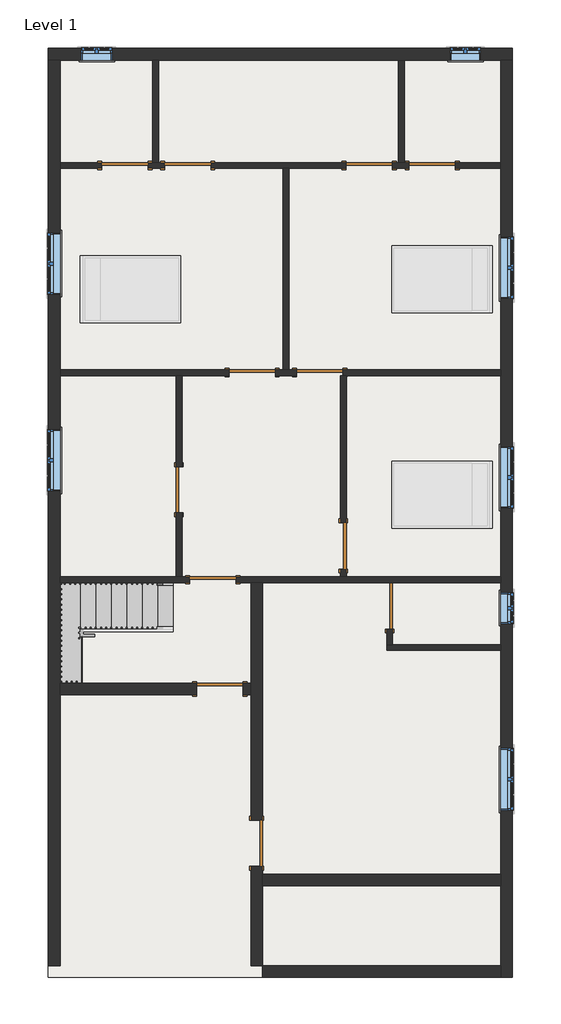
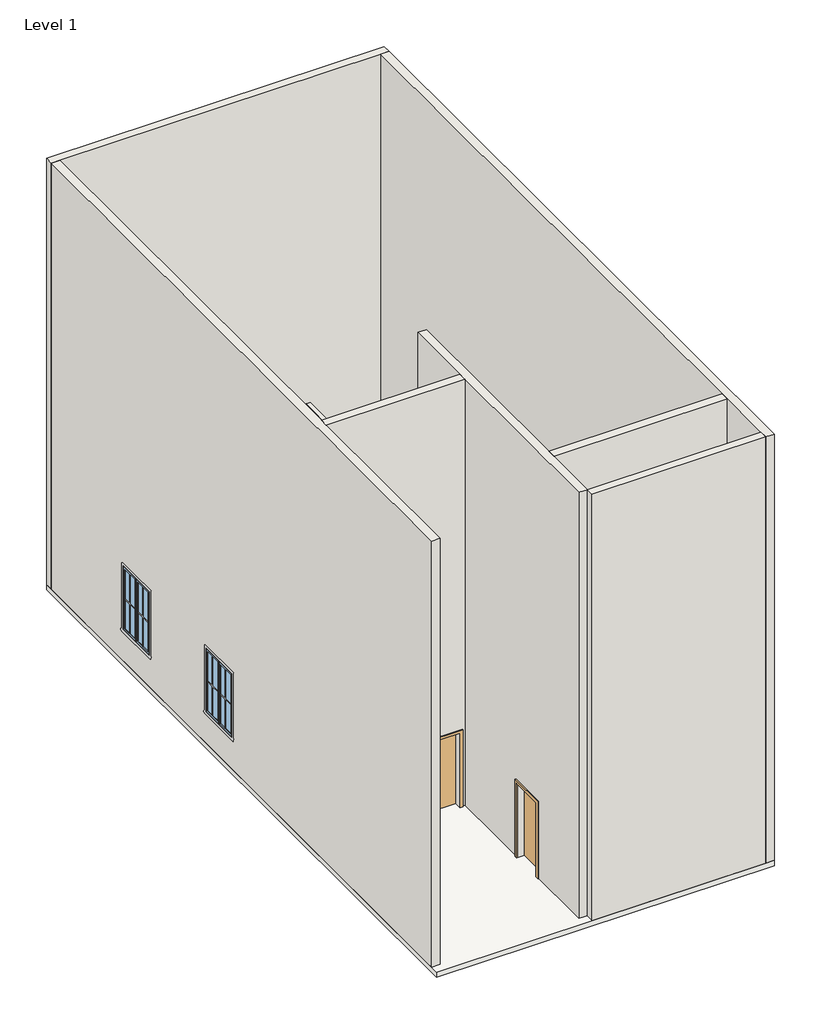
# One storey, part 1 of 2: 17 walls, 12 doors, 8 windows, 1 railing, 1 slab, 1 stair flight.
"""IFC4 building model written with IfcOpenShell, lengths in millimetres."""

from ifc_helpers import new_model, si_unit, frame, origin, origin_with_axes, place, context, project, spatial, polyline, outline, extrude, faceted_brep, transform, mapped, element, save
from components import door_305aa2a5, door_e5f9f3c4, door_0ca8825f, stair_flight_3e22188b, window_c417fced, window_6ca1769e

model = new_model("IFC4")

# Units and contexts
model_context = context("Model", 3, world=origin())
ifc_project = project(units=[si_unit("LENGTHUNIT", "METRE", prefix="MILLI")], contexts=[model_context])

# Site, building, storey
site = spatial("IfcSite", under=ifc_project)
building = spatial("IfcBuilding", under=site)
storey = spatial("IfcBuildingStorey", under=building, Name="Level 1", Elevation=0.0)

# Doors
placement = place(None, origin())
door_shape = door_305aa2a5(model_context)
element("IfcDoor", 1, ObjectType="Single-Flush : 36\" x 84\"", at=placement, inside=storey, context=model_context, shape_type="MappedRepresentation", body=[
    mapped(door_shape, transform((4013.2, 11918.95, 0.0), x_axis=(-1.0, 0.0, 0.0), y_axis=(0.0, -1.0, 0.0), z_axis=(0.0, 0.0, 1.0))),
])
element("IfcDoor", 2, ObjectType="Single-Flush : 36\" x 84\"", at=placement, inside=storey, context=model_context, shape_type="MappedRepresentation", body=[
    mapped(door_shape, transform((8832.85, 11918.95, 0.0), x_axis=(-1.0, 0.0, 0.0), y_axis=(0.0, -1.0, 0.0), z_axis=(0.0, 0.0, 1.0))),
])
element("IfcDoor", 3, ObjectType="Single-Flush : 36\" x 84\"", at=placement, inside=storey, context=model_context, shape_type="MappedRepresentation", body=[
    mapped(door_shape, transform((6616.7, 7842.25, 0.0), x_axis=(-1.0, 0.0, 0.0), y_axis=(0.0, -1.0, 0.0), z_axis=(0.0, 0.0, 1.0))),
])
element("IfcDoor", 4, ObjectType="Single-Flush : 36\" x 84\"", at=placement, inside=storey, context=model_context, shape_type="MappedRepresentation", body=[
    mapped(door_shape, transform((3841.75, 5537.2, 0.0), x_axis=(0.0, -1.0, 0.0), y_axis=(1.0, 0.0, 0.0), z_axis=(0.0, 0.0, 1.0))),
])
door_2_shape = door_e5f9f3c4(model_context)
element("IfcDoor", 5, ObjectType="Single-Flush : 36\" x 84\"", at=placement, inside=storey, context=model_context, shape_type="MappedRepresentation", body=[
    mapped(door_2_shape, transform((2774.95, 11918.95, 0.0), x_axis=(1.0, 0.0, 0.0), y_axis=(0.0, 1.0, 0.0), z_axis=(0.0, 0.0, 1.0))),
])
element("IfcDoor", 6, ObjectType="Single-Flush : 36\" x 84\"", at=placement, inside=storey, context=model_context, shape_type="MappedRepresentation", body=[
    mapped(door_2_shape, transform((7588.25, 11918.95, 0.0), x_axis=(1.0, 0.0, 0.0), y_axis=(0.0, 1.0, 0.0), z_axis=(0.0, 0.0, 1.0))),
])
element("IfcDoor", 7, ObjectType="Single-Flush : 36\" x 84\"", at=placement, inside=storey, context=model_context, shape_type="MappedRepresentation", body=[
    mapped(door_2_shape, transform((5283.2, 7842.25, 0.0), x_axis=(1.0, 0.0, 0.0), y_axis=(0.0, 1.0, 0.0), z_axis=(0.0, 0.0, 1.0))),
])
element("IfcDoor", 8, ObjectType="Single-Flush : 36\" x 84\"", at=placement, inside=storey, context=model_context, shape_type="MappedRepresentation", body=[
    mapped(door_2_shape, transform((4508.5, 3765.55, 0.0), x_axis=(1.0, 0.0, 0.0), y_axis=(0.0, 1.0, 0.0), z_axis=(0.0, 0.0, 1.0))),
])
element("IfcDoor", 9, ObjectType="Single-Flush : 36\" x 84\"", at=placement, inside=storey, context=model_context, shape_type="MappedRepresentation", body=[
    mapped(door_2_shape, transform((7080.25, 4432.3, 0.0), x_axis=(0.0, -1.0, 0.0), y_axis=(1.0, 0.0, 0.0), z_axis=(0.0, 0.0, 1.0))),
])
element("IfcDoor", 10, ObjectType="Single-Flush : 36\" x 84\"", at=placement, inside=storey, context=model_context, shape_type="MappedRepresentation", body=[
    mapped(door_2_shape, transform((7994.65, 3251.2, 0.0), x_axis=(0.0, -1.0, 0.0), y_axis=(1.0, 0.0, 0.0), z_axis=(0.0, 0.0, 1.0))),
])
door_3_shape = door_0ca8825f(model_context)
element("IfcDoor", 11, ObjectType="Single-Flush : 36\" x 84\"", at=placement, inside=storey, context=model_context, shape_type="MappedRepresentation", body=[
    mapped(door_3_shape, transform((4648.2, 1612.9, 0.0), x_axis=(1.0, 0.0, 0.0), y_axis=(0.0, 1.0, 0.0), z_axis=(0.0, 0.0, 1.0))),
])
element("IfcDoor", 12, ObjectType="Single-Flush : 36\" x 84\"", at=placement, inside=storey, context=model_context, shape_type="MappedRepresentation", body=[
    mapped(door_3_shape, transform((5372.1, -1422.4, 0.0), x_axis=(0.0, -1.0, 0.0), y_axis=(1.0, 0.0, 0.0), z_axis=(0.0, 0.0, 1.0))),
])

# Railing
element("IfcRailing", 13, ObjectType="Handrail - Rectangular", at=placement, inside=storey, context=model_context, shape_type="SolidModel", body=[
    faceted_brep([(3727.9146873, 3657.6, 1083.7333333), (3727.9146873, 3657.6, 1025.620221), (3727.9146873, 3708.4, 1025.620221), (3727.9146873, 3708.4, 1083.7333333), (1899.1146873, 3657.6, 2099.7333333), (1885.9510851, 3657.6, 2048.9333333), (1885.9510851, 3708.4, 2048.9333333), (1899.1146873, 3708.4, 2099.7333333), (1549.4, 3657.6, 2099.7333333), (1549.4, 3657.6, 2048.9333333), (1498.6, 3708.4, 2048.9333333), (1498.6, 3708.4, 2099.7333333), (1549.4, 1778.0, 2099.7333333), (1549.4, 1778.0, 2048.9333333), (1498.6, 1727.2, 2048.9333333), (1498.6, 1727.2, 2099.7333333), (1594.3146873, 1778.0, 2099.7333333), (1607.4782895, 1778.0, 2048.9333333), (1607.4782895, 1727.2, 2048.9333333), (1594.3146873, 1727.2, 2099.7333333), (3727.9146873, 1778.0, 3285.0666667), (3727.9146873, 1727.2, 3285.0666667), (3727.9146873, 1727.2, 3226.9535543), (3727.9146873, 1778.0, 3226.9535543)], [[[0, 1, 2, 3]], [[1, 0, 4, 5]], [[2, 1, 5, 6]], [[3, 2, 6, 7]], [[0, 3, 7, 4]], [[5, 4, 8, 9]], [[6, 5, 9, 10]], [[7, 6, 10, 11]], [[4, 7, 11, 8]], [[9, 8, 12, 13]], [[10, 9, 13, 14]], [[11, 10, 14, 15]], [[8, 11, 15, 12]], [[13, 12, 16, 17]], [[14, 13, 17, 18]], [[15, 14, 18, 19]], [[12, 15, 19, 16]], [[20, 21, 22, 23]], [[17, 16, 20, 23]], [[18, 17, 23, 22]], [[19, 18, 22, 21]], [[16, 19, 21, 20]]]),
    extrude(outline(polyline([(3193.1815058, 3667.125), (3182.5981725, 3648.075), (2201.3333333, 3648.075), (2201.3333333, 3667.125), (3193.1815058, 3667.125)])), frame((0.0, 1743.075, 0.0), z_axis=(0.0, 1.0, 0.0), x_axis=(0.0, 0.0, 1.0)), (0.0, 0.0, 1.0), 19.05),
    extrude(outline(polyline([(3136.7370614, 3565.525), (3126.153728, 3546.475), (2201.3333333, 3546.475), (2201.3333333, 3565.525), (3136.7370614, 3565.525)])), frame((0.0, 1743.075, 0.0), z_axis=(0.0, 1.0, 0.0), x_axis=(0.0, 0.0, 1.0)), (0.0, 0.0, 1.0), 19.05),
    extrude(outline(polyline([(3080.2926169, 3463.925), (3069.7092836, 3444.875), (2201.3333333, 3444.875), (2201.3333333, 3463.925), (3080.2926169, 3463.925)])), frame((0.0, 1743.075, 0.0), z_axis=(0.0, 1.0, 0.0), x_axis=(0.0, 0.0, 1.0)), (0.0, 0.0, 1.0), 19.05),
    extrude(outline(polyline([(3023.8481725, 3362.325), (3013.2648391, 3343.275), (2032.0, 3343.275), (2032.0, 3362.325), (3023.8481725, 3362.325)])), frame((0.0, 1743.075, 0.0), z_axis=(0.0, 1.0, 0.0), x_axis=(0.0, 0.0, 1.0)), (0.0, 0.0, 1.0), 19.05),
    extrude(outline(polyline([(2967.403728, 3260.725), (2956.8203947, 3241.675), (2032.0, 3241.675), (2032.0, 3260.725), (2967.403728, 3260.725)])), frame((0.0, 1743.075, 0.0), z_axis=(0.0, 1.0, 0.0), x_axis=(0.0, 0.0, 1.0)), (0.0, 0.0, 1.0), 19.05),
    extrude(outline(polyline([(2910.9592836, 3159.125), (2900.3759503, 3140.075), (2032.0, 3140.075), (2032.0, 3159.125), (2910.9592836, 3159.125)])), frame((0.0, 1743.075, 0.0), z_axis=(0.0, 1.0, 0.0), x_axis=(0.0, 0.0, 1.0)), (0.0, 0.0, 1.0), 19.05),
    extrude(outline(polyline([(2854.5148391, 3057.525), (2843.9315058, 3038.475), (1862.6666667, 3038.475), (1862.6666667, 3057.525), (2854.5148391, 3057.525)])), frame((0.0, 1743.075, 0.0), z_axis=(0.0, 1.0, 0.0), x_axis=(0.0, 0.0, 1.0)), (0.0, 0.0, 1.0), 19.05),
    extrude(outline(polyline([(2798.0703947, 2955.925), (2787.4870614, 2936.875), (1862.6666667, 2936.875), (1862.6666667, 2955.925), (2798.0703947, 2955.925)])), frame((0.0, 1743.075, 0.0), z_axis=(0.0, 1.0, 0.0), x_axis=(0.0, 0.0, 1.0)), (0.0, 0.0, 1.0), 19.05),
    extrude(outline(polyline([(2741.6259503, 2854.325), (2731.0426169, 2835.275), (1862.6666667, 2835.275), (1862.6666667, 2854.325), (2741.6259503, 2854.325)])), frame((0.0, 1743.075, 0.0), z_axis=(0.0, 1.0, 0.0), x_axis=(0.0, 0.0, 1.0)), (0.0, 0.0, 1.0), 19.05),
    extrude(outline(polyline([(2685.1815058, 2752.725), (2674.5981725, 2733.675), (1693.3333333, 2733.675), (1693.3333333, 2752.725), (2685.1815058, 2752.725)])), frame((0.0, 1743.075, 0.0), z_axis=(0.0, 1.0, 0.0), x_axis=(0.0, 0.0, 1.0)), (0.0, 0.0, 1.0), 19.05),
    extrude(outline(polyline([(2628.7370614, 2651.125), (2618.153728, 2632.075), (1693.3333333, 2632.075), (1693.3333333, 2651.125), (2628.7370614, 2651.125)])), frame((0.0, 1743.075, 0.0), z_axis=(0.0, 1.0, 0.0), x_axis=(0.0, 0.0, 1.0)), (0.0, 0.0, 1.0), 19.05),
    extrude(outline(polyline([(2572.2926169, 2549.525), (2561.7092836, 2530.475), (1693.3333333, 2530.475), (1693.3333333, 2549.525), (2572.2926169, 2549.525)])), frame((0.0, 1743.075, 0.0), z_axis=(0.0, 1.0, 0.0), x_axis=(0.0, 0.0, 1.0)), (0.0, 0.0, 1.0), 19.05),
    extrude(outline(polyline([(2515.8481725, 2447.925), (2505.2648391, 2428.875), (1524.0, 2428.875), (1524.0, 2447.925), (2515.8481725, 2447.925)])), frame((0.0, 1743.075, 0.0), z_axis=(0.0, 1.0, 0.0), x_axis=(0.0, 0.0, 1.0)), (0.0, 0.0, 1.0), 19.05),
    extrude(outline(polyline([(2459.403728, 2346.325), (2448.8203947, 2327.275), (1524.0, 2327.275), (1524.0, 2346.325), (2459.403728, 2346.325)])), frame((0.0, 1743.075, 0.0), z_axis=(0.0, 1.0, 0.0), x_axis=(0.0, 0.0, 1.0)), (0.0, 0.0, 1.0), 19.05),
    extrude(outline(polyline([(2402.9592836, 2244.725), (2392.3759503, 2225.675), (1524.0, 2225.675), (1524.0, 2244.725), (2402.9592836, 2244.725)])), frame((0.0, 1743.075, 0.0), z_axis=(0.0, 1.0, 0.0), x_axis=(0.0, 0.0, 1.0)), (0.0, 0.0, 1.0), 19.05),
    extrude(outline(polyline([(2346.5148391, 2143.125), (2335.9315058, 2124.075), (1354.6666667, 2124.075), (1354.6666667, 2143.125), (2346.5148391, 2143.125)])), frame((0.0, 1743.075, 0.0), z_axis=(0.0, 1.0, 0.0), x_axis=(0.0, 0.0, 1.0)), (0.0, 0.0, 1.0), 19.05),
    extrude(outline(polyline([(2290.0703947, 2041.525), (2279.4870614, 2022.475), (1354.6666667, 2022.475), (1354.6666667, 2041.525), (2290.0703947, 2041.525)])), frame((0.0, 1743.075, 0.0), z_axis=(0.0, 1.0, 0.0), x_axis=(0.0, 0.0, 1.0)), (0.0, 0.0, 1.0), 19.05),
    extrude(outline(polyline([(2233.6259503, 1939.925), (2223.0426169, 1920.875), (1354.6666667, 1920.875), (1354.6666667, 1939.925), (2233.6259503, 1939.925)])), frame((0.0, 1743.075, 0.0), z_axis=(0.0, 1.0, 0.0), x_axis=(0.0, 0.0, 1.0)), (0.0, 0.0, 1.0), 19.05),
    extrude(outline(polyline([(2177.1815058, 1838.325), (2166.5981725, 1819.275), (1185.3333333, 1819.275), (1185.3333333, 1838.325), (2177.1815058, 1838.325)])), frame((0.0, 1743.075, 0.0), z_axis=(0.0, 1.0, 0.0), x_axis=(0.0, 0.0, 1.0)), (0.0, 0.0, 1.0), 19.05),
    extrude(outline(polyline([(2120.7370614, 1736.725), (2110.153728, 1717.675), (1185.3333333, 1717.675), (1185.3333333, 1736.725), (2120.7370614, 1736.725)])), frame((0.0, 1743.075, 0.0), z_axis=(0.0, 1.0, 0.0), x_axis=(0.0, 0.0, 1.0)), (0.0, 0.0, 1.0), 19.05),
    extrude(outline(polyline([(2064.2926169, 1635.125), (2053.7092836, 1616.075), (1185.3333333, 1616.075), (1185.3333333, 1635.125), (2064.2926169, 1635.125)])), frame((0.0, 1743.075, 0.0), z_axis=(0.0, 1.0, 0.0), x_axis=(0.0, 0.0, 1.0)), (0.0, 0.0, 1.0), 19.05),
    extrude(outline(polyline([(1514.475, 1863.725), (1533.525, 1863.725), (1533.525, 1844.675), (1514.475, 1844.675), (1514.475, 1863.725)])), frame((0.0, 0.0, 1185.3333333), z_axis=(0.0, 0.0, 1.0), x_axis=(1.0, 0.0, 0.0)), (0.0, 0.0, 1.0), 863.6),
    extrude(outline(polyline([(1514.475, 1965.325), (1533.525, 1965.325), (1533.525, 1946.275), (1514.475, 1946.275), (1514.475, 1965.325)])), frame((0.0, 0.0, 1185.3333333), z_axis=(0.0, 0.0, 1.0), x_axis=(1.0, 0.0, 0.0)), (0.0, 0.0, 1.0), 863.6),
    extrude(outline(polyline([(1514.475, 2066.925), (1533.525, 2066.925), (1533.525, 2047.875), (1514.475, 2047.875), (1514.475, 2066.925)])), frame((0.0, 0.0, 1185.3333333), z_axis=(0.0, 0.0, 1.0), x_axis=(1.0, 0.0, 0.0)), (0.0, 0.0, 1.0), 863.6),
    extrude(outline(polyline([(1514.475, 2168.525), (1533.525, 2168.525), (1533.525, 2149.475), (1514.475, 2149.475), (1514.475, 2168.525)])), frame((0.0, 0.0, 1185.3333333), z_axis=(0.0, 0.0, 1.0), x_axis=(1.0, 0.0, 0.0)), (0.0, 0.0, 1.0), 863.6),
    extrude(outline(polyline([(1514.475, 2270.125), (1533.525, 2270.125), (1533.525, 2251.075), (1514.475, 2251.075), (1514.475, 2270.125)])), frame((0.0, 0.0, 1185.3333333), z_axis=(0.0, 0.0, 1.0), x_axis=(1.0, 0.0, 0.0)), (0.0, 0.0, 1.0), 863.6),
    extrude(outline(polyline([(1514.475, 2371.725), (1533.525, 2371.725), (1533.525, 2352.675), (1514.475, 2352.675), (1514.475, 2371.725)])), frame((0.0, 0.0, 1185.3333333), z_axis=(0.0, 0.0, 1.0), x_axis=(1.0, 0.0, 0.0)), (0.0, 0.0, 1.0), 863.6),
    extrude(outline(polyline([(1514.475, 2473.325), (1533.525, 2473.325), (1533.525, 2454.275), (1514.475, 2454.275), (1514.475, 2473.325)])), frame((0.0, 0.0, 1185.3333333), z_axis=(0.0, 0.0, 1.0), x_axis=(1.0, 0.0, 0.0)), (0.0, 0.0, 1.0), 863.6),
    extrude(outline(polyline([(1514.475, 2574.925), (1533.525, 2574.925), (1533.525, 2555.875), (1514.475, 2555.875), (1514.475, 2574.925)])), frame((0.0, 0.0, 1185.3333333), z_axis=(0.0, 0.0, 1.0), x_axis=(1.0, 0.0, 0.0)), (0.0, 0.0, 1.0), 863.6),
    extrude(outline(polyline([(1514.475, 2676.525), (1533.525, 2676.525), (1533.525, 2657.475), (1514.475, 2657.475), (1514.475, 2676.525)])), frame((0.0, 0.0, 1185.3333333), z_axis=(0.0, 0.0, 1.0), x_axis=(1.0, 0.0, 0.0)), (0.0, 0.0, 1.0), 863.6),
    extrude(outline(polyline([(1514.475, 2778.125), (1533.525, 2778.125), (1533.525, 2759.075), (1514.475, 2759.075), (1514.475, 2778.125)])), frame((0.0, 0.0, 1185.3333333), z_axis=(0.0, 0.0, 1.0), x_axis=(1.0, 0.0, 0.0)), (0.0, 0.0, 1.0), 863.6),
    extrude(outline(polyline([(1514.475, 2879.725), (1533.525, 2879.725), (1533.525, 2860.675), (1514.475, 2860.675), (1514.475, 2879.725)])), frame((0.0, 0.0, 1185.3333333), z_axis=(0.0, 0.0, 1.0), x_axis=(1.0, 0.0, 0.0)), (0.0, 0.0, 1.0), 863.6),
    extrude(outline(polyline([(1514.475, 2981.325), (1533.525, 2981.325), (1533.525, 2962.275), (1514.475, 2962.275), (1514.475, 2981.325)])), frame((0.0, 0.0, 1185.3333333), z_axis=(0.0, 0.0, 1.0), x_axis=(1.0, 0.0, 0.0)), (0.0, 0.0, 1.0), 863.6),
    extrude(outline(polyline([(1514.475, 3082.925), (1533.525, 3082.925), (1533.525, 3063.875), (1514.475, 3063.875), (1514.475, 3082.925)])), frame((0.0, 0.0, 1185.3333333), z_axis=(0.0, 0.0, 1.0), x_axis=(1.0, 0.0, 0.0)), (0.0, 0.0, 1.0), 863.6),
    extrude(outline(polyline([(1514.475, 3184.525), (1533.525, 3184.525), (1533.525, 3165.475), (1514.475, 3165.475), (1514.475, 3184.525)])), frame((0.0, 0.0, 1185.3333333), z_axis=(0.0, 0.0, 1.0), x_axis=(1.0, 0.0, 0.0)), (0.0, 0.0, 1.0), 863.6),
    extrude(outline(polyline([(1514.475, 3286.125), (1533.525, 3286.125), (1533.525, 3267.075), (1514.475, 3267.075), (1514.475, 3286.125)])), frame((0.0, 0.0, 1185.3333333), z_axis=(0.0, 0.0, 1.0), x_axis=(1.0, 0.0, 0.0)), (0.0, 0.0, 1.0), 863.6),
    extrude(outline(polyline([(1514.475, 3387.725), (1533.525, 3387.725), (1533.525, 3368.675), (1514.475, 3368.675), (1514.475, 3387.725)])), frame((0.0, 0.0, 1185.3333333), z_axis=(0.0, 0.0, 1.0), x_axis=(1.0, 0.0, 0.0)), (0.0, 0.0, 1.0), 863.6),
    extrude(outline(polyline([(1514.475, 3489.325), (1533.525, 3489.325), (1533.525, 3470.275), (1514.475, 3470.275), (1514.475, 3489.325)])), frame((0.0, 0.0, 1185.3333333), z_axis=(0.0, 0.0, 1.0), x_axis=(1.0, 0.0, 0.0)), (0.0, 0.0, 1.0), 863.6),
    extrude(outline(polyline([(1514.475, 3590.925), (1533.525, 3590.925), (1533.525, 3571.875), (1514.475, 3571.875), (1514.475, 3590.925)])), frame((0.0, 0.0, 1185.3333333), z_axis=(0.0, 0.0, 1.0), x_axis=(1.0, 0.0, 0.0)), (0.0, 0.0, 1.0), 863.6),
    extrude(outline(polyline([(1603.8396873, 3692.525), (1603.8396873, 3673.475), (1584.7896873, 3673.475), (1584.7896873, 3692.525), (1603.8396873, 3692.525)])), frame((0.0, 0.0, 1185.3333333), z_axis=(0.0, 0.0, 1.0), x_axis=(1.0, 0.0, 0.0)), (0.0, 0.0, 1.0), 863.6),
    extrude(outline(polyline([(1705.4396873, 3692.525), (1705.4396873, 3673.475), (1686.3896873, 3673.475), (1686.3896873, 3692.525), (1705.4396873, 3692.525)])), frame((0.0, 0.0, 1185.3333333), z_axis=(0.0, 0.0, 1.0), x_axis=(1.0, 0.0, 0.0)), (0.0, 0.0, 1.0), 863.6),
    extrude(outline(polyline([(1807.0396873, 3692.525), (1807.0396873, 3673.475), (1787.9896873, 3673.475), (1787.9896873, 3692.525), (1807.0396873, 3692.525)])), frame((0.0, 0.0, 1185.3333333), z_axis=(0.0, 0.0, 1.0), x_axis=(1.0, 0.0, 0.0)), (0.0, 0.0, 1.0), 863.6),
    extrude(outline(polyline([(2036.3285543, 1908.6396873), (2046.9118876, 1889.5896873), (1185.3333333, 1889.5896873), (1185.3333333, 1908.6396873), (2036.3285543, 1908.6396873)])), frame((0.0, 3673.475, 0.0), z_axis=(0.0, 1.0, 0.0), x_axis=(0.0, 0.0, 1.0)), (0.0, 0.0, 1.0), 19.05),
    extrude(outline(polyline([(1979.8841099, 2010.2396873), (1990.4674432, 1991.1896873), (1016.0, 1991.1896873), (1016.0, 2010.2396873), (1979.8841099, 2010.2396873)])), frame((0.0, 3673.475, 0.0), z_axis=(0.0, 1.0, 0.0), x_axis=(0.0, 0.0, 1.0)), (0.0, 0.0, 1.0), 19.05),
    extrude(outline(polyline([(1923.4396654, 2111.8396873), (1934.0229988, 2092.7896873), (1016.0, 2092.7896873), (1016.0, 2111.8396873), (1923.4396654, 2111.8396873)])), frame((0.0, 3673.475, 0.0), z_axis=(0.0, 1.0, 0.0), x_axis=(0.0, 0.0, 1.0)), (0.0, 0.0, 1.0), 19.05),
    extrude(outline(polyline([(1866.995221, 2213.4396873), (1877.5785543, 2194.3896873), (1016.0, 2194.3896873), (1016.0, 2213.4396873), (1866.995221, 2213.4396873)])), frame((0.0, 3673.475, 0.0), z_axis=(0.0, 1.0, 0.0), x_axis=(0.0, 0.0, 1.0)), (0.0, 0.0, 1.0), 19.05),
    extrude(outline(polyline([(1810.5507765, 2315.0396873), (1821.1341099, 2295.9896873), (846.6666667, 2295.9896873), (846.6666667, 2315.0396873), (1810.5507765, 2315.0396873)])), frame((0.0, 3673.475, 0.0), z_axis=(0.0, 1.0, 0.0), x_axis=(0.0, 0.0, 1.0)), (0.0, 0.0, 1.0), 19.05),
    extrude(outline(polyline([(1754.1063321, 2416.6396873), (1764.6896654, 2397.5896873), (846.6666667, 2397.5896873), (846.6666667, 2416.6396873), (1754.1063321, 2416.6396873)])), frame((0.0, 3673.475, 0.0), z_axis=(0.0, 1.0, 0.0), x_axis=(0.0, 0.0, 1.0)), (0.0, 0.0, 1.0), 19.05),
    extrude(outline(polyline([(1697.6618876, 2518.2396873), (1708.245221, 2499.1896873), (846.6666667, 2499.1896873), (846.6666667, 2518.2396873), (1697.6618876, 2518.2396873)])), frame((0.0, 3673.475, 0.0), z_axis=(0.0, 1.0, 0.0), x_axis=(0.0, 0.0, 1.0)), (0.0, 0.0, 1.0), 19.05),
    extrude(outline(polyline([(1641.2174432, 2619.8396873), (1651.8007765, 2600.7896873), (677.3333333, 2600.7896873), (677.3333333, 2619.8396873), (1641.2174432, 2619.8396873)])), frame((0.0, 3673.475, 0.0), z_axis=(0.0, 1.0, 0.0), x_axis=(0.0, 0.0, 1.0)), (0.0, 0.0, 1.0), 19.05),
    extrude(outline(polyline([(1584.7729988, 2721.4396873), (1595.3563321, 2702.3896873), (677.3333333, 2702.3896873), (677.3333333, 2721.4396873), (1584.7729988, 2721.4396873)])), frame((0.0, 3673.475, 0.0), z_axis=(0.0, 1.0, 0.0), x_axis=(0.0, 0.0, 1.0)), (0.0, 0.0, 1.0), 19.05),
    extrude(outline(polyline([(1528.3285543, 2823.0396873), (1538.9118876, 2803.9896873), (677.3333333, 2803.9896873), (677.3333333, 2823.0396873), (1528.3285543, 2823.0396873)])), frame((0.0, 3673.475, 0.0), z_axis=(0.0, 1.0, 0.0), x_axis=(0.0, 0.0, 1.0)), (0.0, 0.0, 1.0), 19.05),
    extrude(outline(polyline([(1471.8841099, 2924.6396873), (1482.4674432, 2905.5896873), (508.0, 2905.5896873), (508.0, 2924.6396873), (1471.8841099, 2924.6396873)])), frame((0.0, 3673.475, 0.0), z_axis=(0.0, 1.0, 0.0), x_axis=(0.0, 0.0, 1.0)), (0.0, 0.0, 1.0), 19.05),
    extrude(outline(polyline([(1415.4396654, 3026.2396873), (1426.0229988, 3007.1896873), (508.0, 3007.1896873), (508.0, 3026.2396873), (1415.4396654, 3026.2396873)])), frame((0.0, 3673.475, 0.0), z_axis=(0.0, 1.0, 0.0), x_axis=(0.0, 0.0, 1.0)), (0.0, 0.0, 1.0), 19.05),
    extrude(outline(polyline([(1358.995221, 3127.8396873), (1369.5785543, 3108.7896873), (508.0, 3108.7896873), (508.0, 3127.8396873), (1358.995221, 3127.8396873)])), frame((0.0, 3673.475, 0.0), z_axis=(0.0, 1.0, 0.0), x_axis=(0.0, 0.0, 1.0)), (0.0, 0.0, 1.0), 19.05),
    extrude(outline(polyline([(1302.5507765, 3229.4396873), (1313.1341099, 3210.3896873), (338.6666667, 3210.3896873), (338.6666667, 3229.4396873), (1302.5507765, 3229.4396873)])), frame((0.0, 3673.475, 0.0), z_axis=(0.0, 1.0, 0.0), x_axis=(0.0, 0.0, 1.0)), (0.0, 0.0, 1.0), 19.05),
    extrude(outline(polyline([(1246.1063321, 3331.0396873), (1256.6896654, 3311.9896873), (338.6666667, 3311.9896873), (338.6666667, 3331.0396873), (1246.1063321, 3331.0396873)])), frame((0.0, 3673.475, 0.0), z_axis=(0.0, 1.0, 0.0), x_axis=(0.0, 0.0, 1.0)), (0.0, 0.0, 1.0), 19.05),
    extrude(outline(polyline([(1189.6618876, 3432.6396873), (1200.245221, 3413.5896873), (338.6666667, 3413.5896873), (338.6666667, 3432.6396873), (1189.6618876, 3432.6396873)])), frame((0.0, 3673.475, 0.0), z_axis=(0.0, 1.0, 0.0), x_axis=(0.0, 0.0, 1.0)), (0.0, 0.0, 1.0), 19.05),
    extrude(outline(polyline([(1133.2174432, 3534.2396873), (1143.8007765, 3515.1896873), (169.3333333, 3515.1896873), (169.3333333, 3534.2396873), (1133.2174432, 3534.2396873)])), frame((0.0, 3673.475, 0.0), z_axis=(0.0, 1.0, 0.0), x_axis=(0.0, 0.0, 1.0)), (0.0, 0.0, 1.0), 19.05),
    extrude(outline(polyline([(1076.7729988, 3635.8396873), (1087.3563321, 3616.7896873), (169.3333333, 3616.7896873), (169.3333333, 3635.8396873), (1076.7729988, 3635.8396873)])), frame((0.0, 3673.475, 0.0), z_axis=(0.0, 1.0, 0.0), x_axis=(0.0, 0.0, 1.0)), (0.0, 0.0, 1.0), 19.05),
    extrude(outline(polyline([(1514.475, 1762.125), (1533.525, 1762.125), (1533.525, 1743.075), (1514.475, 1743.075), (1514.475, 1762.125)])), frame((0.0, 0.0, 1185.3333333), z_axis=(0.0, 0.0, 1.0), x_axis=(1.0, 0.0, 0.0)), (0.0, 0.0, 1.0), 863.6),
    extrude(outline(polyline([(1533.525, 3692.525), (1533.525, 3673.475), (1514.475, 3673.475), (1514.475, 3692.525), (1533.525, 3692.525)])), frame((0.0, 0.0, 1185.3333333), z_axis=(0.0, 0.0, 1.0), x_axis=(1.0, 0.0, 0.0)), (0.0, 0.0, 1.0), 863.6),
    extrude(outline(polyline([(3226.9535543, 3727.9146873), (3216.370221, 3708.8646873), (2201.3333333, 3708.8646873), (2201.3333333, 3727.9146873), (3226.9535543, 3727.9146873)])), frame((0.0, 1743.075, 0.0), z_axis=(0.0, 1.0, 0.0), x_axis=(0.0, 0.0, 1.0)), (0.0, 0.0, 1.0), 19.05),
    extrude(outline(polyline([(1025.620221, 3727.9146873), (1036.2035543, 3708.8646873), (169.3333333, 3708.8646873), (169.3333333, 3727.9146873), (1025.620221, 3727.9146873)])), frame((0.0, 3673.475, 0.0), z_axis=(0.0, 1.0, 0.0), x_axis=(0.0, 0.0, 1.0)), (0.0, 0.0, 1.0), 19.05),
])

# Slab
element("IfcSlab", 14, ObjectType="Generic - 12\"", at=placement, inside=storey, context=model_context, shape_type="SweptSolid", body=[
    extrude(outline(polyline([(10414.0, 14224.0), (10414.0, -4064.0), (1270.0, -4064.0), (1270.0, 14224.0), (10414.0, 14224.0)])), frame((0.0, 0.0, -152.4), z_axis=(0.0, 0.0, 1.0), x_axis=(1.0, 0.0, 0.0)), (0.0, 0.0, 1.0), 152.4),
])

# Stair flight
stair_flight_shape = stair_flight_3e22188b(model_context)
element("IfcStairFlight", 15, ObjectType="2\" Tread 1\" Nosing 1/4\" Riser", at=placement, inside=storey, context=model_context, shape_type="MappedRepresentation", body=[
    mapped(stair_flight_shape, transform((0.0, 0.0, 0.0), x_axis=(1.0, 0.0, 0.0), y_axis=(0.0, 1.0, 0.0), z_axis=(0.0, 0.0, 1.0))),
])

# Walls
element("IfcWall", 16, ObjectType="Generic - 5\"", at=placement, inside=storey, context=model_context, shape_type="Brep", body=[
    faceted_brep([(8045.45, 11861.8, 0.0), (8375.65, 11861.8, 0.0), (8375.65, 11861.8, 2133.6), (9290.05, 11861.8, 2133.6), (9290.05, 11861.8, 0.0), (10185.4, 11861.8, 0.0), (10185.4, 11861.8, 2895.6), (6007.1, 11861.8, 2895.6), (5892.8, 11861.8, 2895.6), (1498.6, 11861.8, 2895.6), (1498.6, 11861.8, 0.0), (2317.75, 11861.8, 0.0), (2317.75, 11861.8, 2133.6), (3232.15, 11861.8, 2133.6), (3232.15, 11861.8, 0.0), (3556.0, 11861.8, 0.0), (3556.0, 11861.8, 2133.6), (4470.4, 11861.8, 2133.6), (4470.4, 11861.8, 0.0), (5892.8, 11861.8, 0.0), (6007.1, 11861.8, 0.0), (7131.05, 11861.8, 0.0), (7131.05, 11861.8, 2133.6), (8045.45, 11861.8, 2133.6), (8375.65, 11976.1, 2133.6), (8375.65, 11976.1, 0.0), (8280.4, 11976.1, 0.0), (8166.1, 11976.1, 0.0), (8045.45, 11976.1, 0.0), (8045.45, 11976.1, 2133.6), (7131.05, 11976.1, 2133.6), (7131.05, 11976.1, 0.0), (4470.4, 11976.1, 0.0), (4470.4, 11976.1, 2133.6), (3556.0, 11976.1, 2133.6), (3556.0, 11976.1, 0.0), (3441.7, 11976.1, 0.0), (3327.4, 11976.1, 0.0), (3232.15, 11976.1, 0.0), (3232.15, 11976.1, 2133.6), (2317.75, 11976.1, 2133.6), (2317.75, 11976.1, 0.0), (1498.6, 11976.1, 0.0), (1498.6, 11976.1, 2895.6), (3327.4, 11976.1, 2895.6), (3441.7, 11976.1, 2895.6), (8166.1, 11976.1, 2895.6), (8280.4, 11976.1, 2895.6), (10185.4, 11976.1, 2895.6), (10185.4, 11976.1, 0.0), (9290.05, 11976.1, 0.0), (9290.05, 11976.1, 2133.6)], [[[0, 1, 2, 3, 4, 5, 6, 7, 8, 9, 10, 11, 12, 13, 14, 15, 16, 17, 18, 19, 20, 21, 22, 23]], [[24, 25, 26, 27, 28, 29, 30, 31, 32, 33, 34, 35, 36, 37, 38, 39, 40, 41, 42, 43, 44, 45, 46, 47, 48, 49, 50, 51]], [[11, 10, 42, 41]], [[15, 14, 38, 37, 36, 35]], [[21, 20, 19, 18, 32, 31]], [[50, 49, 5, 4]], [[28, 27, 26, 25, 1, 0]], [[6, 5, 49, 48]], [[10, 9, 43, 42]], [[16, 15, 35, 34]], [[17, 16, 34, 33]], [[18, 17, 33, 32]], [[39, 38, 14, 13]], [[40, 39, 13, 12]], [[41, 40, 12, 11]], [[29, 28, 0, 23]], [[30, 29, 23, 22]], [[31, 30, 22, 21]], [[2, 1, 25, 24]], [[3, 2, 24, 51]], [[4, 3, 51, 50]], [[9, 8, 7, 6, 48, 47, 46, 45, 44, 43]]]),
])
element("IfcWall", 17, ObjectType="Generic - 5\"", at=placement, inside=storey, context=model_context, shape_type="Brep", body=[
    faceted_brep([(5740.4, 7785.1, 0.0), (6159.5, 7785.1, 0.0), (6159.5, 7785.1, 2133.6), (7073.9, 7785.1, 2133.6), (7073.9, 7785.1, 0.0), (7137.4, 7785.1, 0.0), (10185.4, 7785.1, 0.0), (10185.4, 7785.1, 2895.6), (7137.4, 7785.1, 2895.6), (7023.1, 7785.1, 2895.6), (3898.9, 7785.1, 2895.6), (3784.6, 7785.1, 2895.6), (1498.6, 7785.1, 2895.6), (1498.6, 7785.1, 0.0), (3784.6, 7785.1, 0.0), (3898.9, 7785.1, 0.0), (4826.0, 7785.1, 0.0), (4826.0, 7785.1, 2133.6), (5740.4, 7785.1, 2133.6), (6159.5, 7899.4, 2133.6), (6159.5, 7899.4, 0.0), (6007.1, 7899.4, 0.0), (5892.8, 7899.4, 0.0), (5740.4, 7899.4, 0.0), (5740.4, 7899.4, 2133.6), (4826.0, 7899.4, 2133.6), (4826.0, 7899.4, 0.0), (1498.6, 7899.4, 0.0), (1498.6, 7899.4, 2895.6), (5892.8, 7899.4, 2895.6), (6007.1, 7899.4, 2895.6), (10185.4, 7899.4, 2895.6), (10185.4, 7899.4, 0.0), (7073.9, 7899.4, 0.0), (7073.9, 7899.4, 2133.6)], [[[0, 1, 2, 3, 4, 5, 6, 7, 8, 9, 10, 11, 12, 13, 14, 15, 16, 17, 18]], [[19, 20, 21, 22, 23, 24, 25, 26, 27, 28, 29, 30, 31, 32, 33, 34]], [[16, 15, 14, 13, 27, 26]], [[33, 32, 6, 5, 4]], [[23, 22, 21, 20, 1, 0]], [[7, 6, 32, 31]], [[13, 12, 28, 27]], [[24, 23, 0, 18]], [[25, 24, 18, 17]], [[26, 25, 17, 16]], [[2, 1, 20, 19]], [[3, 2, 19, 34]], [[4, 3, 34, 33]], [[12, 11, 10, 9, 8, 7, 31, 30, 29, 28]]]),
])
element("IfcWall", 18, ObjectType="Generic - 5\"", at=placement, inside=storey, context=model_context, shape_type="SweptSolid", body=[
    extrude(outline(polyline([(5080.0, 2133.6), (5080.0, 0.0), (3822.7, 0.0), (3822.7, 2895.6), (7785.1, 2895.6), (7785.1, 0.0), (5994.4, 0.0), (5994.4, 2133.6), (5080.0, 2133.6)])), frame((3784.6, 0.0, 0.0), z_axis=(1.0, 0.0, 0.0), x_axis=(0.0, 1.0, 0.0)), (0.0, 0.0, 1.0), 114.3),
])
element("IfcWall", 19, ObjectType="Generic - 5\"", at=placement, inside=storey, context=model_context, shape_type="Brep", body=[
    faceted_brep([(4965.7, 3708.4, 2133.6), (4965.7, 3708.4, 0.0), (5257.8, 3708.4, 0.0), (5486.4, 3708.4, 0.0), (10185.4, 3708.4, 0.0), (10185.4, 3708.4, 2895.6), (8051.8, 3708.4, 2895.6), (7937.5, 3708.4, 2895.6), (1498.6, 3708.4, 2895.6), (1498.6, 3708.4, 0.0), (4051.3, 3708.4, 0.0), (4051.3, 3708.4, 2133.6), (10185.4, 3822.7, 0.0), (7137.4, 3822.7, 0.0), (7023.1, 3822.7, 0.0), (4965.7, 3822.7, 0.0), (4965.7, 3822.7, 2133.6), (4051.3, 3822.7, 2133.6), (4051.3, 3822.7, 0.0), (3898.9, 3822.7, 0.0), (3784.6, 3822.7, 0.0), (1498.6, 3822.7, 0.0), (1498.6, 3822.7, 2895.6), (3784.6, 3822.7, 2895.6), (3898.9, 3822.7, 2895.6), (7023.1, 3822.7, 2895.6), (7137.4, 3822.7, 2895.6), (10185.4, 3822.7, 2895.6)], [[[0, 1, 2, 3, 4, 5, 6, 7, 8, 9, 10, 11]], [[12, 13, 14, 15, 16, 17, 18, 19, 20, 21, 22, 23, 24, 25, 26, 27]], [[10, 9, 21, 20, 19, 18]], [[4, 3, 2, 1, 15, 14, 13, 12]], [[5, 4, 12, 27]], [[9, 8, 22, 21]], [[16, 15, 1, 0]], [[17, 16, 0, 11]], [[18, 17, 11, 10]], [[8, 7, 6, 5, 27, 26, 25, 24, 23, 22]]]),
])
element("IfcWall", 20, ObjectType="Generic - 5\"", at=placement, inside=storey, context=model_context, shape_type="Brep", body=[
    faceted_brep([(10185.4, 2489.2, 0.0), (8051.8, 2489.2, 0.0), (7937.5, 2489.2, 0.0), (7937.5, 2489.2, 2895.6), (8051.8, 2489.2, 2895.6), (10185.4, 2489.2, 2895.6), (10185.4, 2374.9, 0.0), (10185.4, 2374.9, 2895.6), (7937.5, 2374.9, 2895.6), (7937.5, 2374.9, 0.0)], [[[0, 1, 2, 3, 4, 5]], [[6, 7, 8, 9]], [[2, 1, 0, 6, 9]], [[0, 5, 7, 6]], [[3, 2, 9, 8]], [[5, 4, 3, 8, 7]]]),
])
element("IfcWall", 21, ObjectType="Generic - 5\"", at=placement, inside=storey, context=model_context, shape_type="SweptSolid", body=[
    extrude(outline(polyline([(2489.2, 0.0), (2489.2, 2895.6), (3708.4, 2895.6), (3708.4, 2133.6), (2794.0, 2133.6), (2794.0, 0.0), (2489.2, 0.0)])), frame((7937.5, 0.0, 0.0), z_axis=(1.0, 0.0, 0.0), x_axis=(0.0, 1.0, 0.0)), (0.0, 0.0, 1.0), 114.3),
])
element("IfcWall", 22, ObjectType="Generic - 5\"", at=placement, inside=storey, context=model_context, shape_type="Brep", body=[
    faceted_brep([(7023.1, 3975.1, 2133.6), (7023.1, 3975.1, 0.0), (7023.1, 3822.7, 0.0), (7023.1, 3822.7, 2895.6), (7023.1, 7785.1, 2895.6), (7023.1, 7785.1, 0.0), (7023.1, 4889.5, 0.0), (7023.1, 4889.5, 2133.6), (7137.4, 3822.7, 0.0), (7137.4, 3975.1, 0.0), (7137.4, 3975.1, 2133.6), (7137.4, 4889.5, 2133.6), (7137.4, 4889.5, 0.0), (7137.4, 7785.1, 0.0), (7137.4, 7785.1, 2895.6), (7137.4, 3822.7, 2895.6), (7073.9, 7785.1, 0.0)], [[[0, 1, 2, 3, 4, 5, 6, 7]], [[8, 9, 10, 11, 12, 13, 14, 15]], [[6, 5, 16, 13, 12]], [[2, 1, 9, 8]], [[5, 4, 14, 13, 16]], [[3, 2, 8, 15]], [[10, 9, 1, 0]], [[11, 10, 0, 7]], [[12, 11, 7, 6]], [[4, 3, 15, 14]]]),
])
element("IfcWall", 23, ObjectType="Generic - 5\"", at=placement, inside=storey, context=model_context, shape_type="SweptSolid", body=[
    extrude(outline(polyline([(3327.4, 11976.1), (3327.4, 13995.4), (3441.7, 13995.4), (3441.7, 11976.1), (3327.4, 11976.1)])), origin_with_axes(), (0.0, 0.0, 1.0), 2895.6),
])
element("IfcWall", 24, ObjectType="Generic - 5\"", at=placement, inside=storey, context=model_context, shape_type="SweptSolid", body=[
    extrude(outline(polyline([(8166.1, 11976.1), (8166.1, 13995.4), (8280.4, 13995.4), (8280.4, 11976.1), (8166.1, 11976.1)])), origin_with_axes(), (0.0, 0.0, 1.0), 2895.6),
])
element("IfcWall", 25, ObjectType="Generic - 5\"", at=placement, inside=storey, context=model_context, shape_type="SweptSolid", body=[
    extrude(outline(polyline([(5892.8, 7899.4), (5892.8, 11861.8), (6007.1, 11861.8), (6007.1, 7899.4), (5892.8, 7899.4)])), origin_with_axes(), (0.0, 0.0, 1.0), 2895.6),
])
element("IfcWall", 26, ObjectType="Generic - 8\"", at=placement, inside=storey, context=model_context, shape_type="Brep", body=[
    faceted_brep([(1270.0, 13995.4, 0.0), (1498.6, 13995.4, 0.0), (3327.4, 13995.4, 0.0), (3441.7, 13995.4, 0.0), (8166.1, 13995.4, 0.0), (8280.4, 13995.4, 0.0), (10185.4, 13995.4, 0.0), (10414.0, 13995.4, 0.0), (10414.0, 13995.4, 12192.0), (10185.4, 13995.4, 12192.0), (1498.6, 13995.4, 12192.0), (1270.0, 13995.4, 12192.0), (9791.7, 13995.4, 1828.8), (9791.7, 13995.4, 914.4), (9182.1, 13995.4, 914.4), (9182.1, 13995.4, 1828.8), (2527.3, 13995.4, 1828.8), (2527.3, 13995.4, 914.4), (1917.7, 13995.4, 914.4), (1917.7, 13995.4, 1828.8), (1270.0, 14224.0, 0.0), (1270.0, 14224.0, 12192.0), (10414.0, 14224.0, 12192.0), (10414.0, 14224.0, 0.0), (9791.7, 14224.0, 1828.8), (9182.1, 14224.0, 1828.8), (9182.1, 14224.0, 914.4), (9791.7, 14224.0, 914.4), (2527.3, 14224.0, 1828.8), (1917.7, 14224.0, 1828.8), (1917.7, 14224.0, 914.4), (2527.3, 14224.0, 914.4)], [[[0, 1, 2, 3, 4, 5, 6, 7, 8, 9, 10, 11], [12, 13, 14, 15], [16, 17, 18, 19]], [[20, 21, 22, 23], [24, 25, 26, 27], [28, 29, 30, 31]], [[7, 6, 5, 4, 3, 2, 1, 0, 20, 23]], [[8, 7, 23, 22]], [[0, 11, 21, 20]], [[13, 12, 24, 27]], [[14, 13, 27, 26]], [[15, 14, 26, 25]], [[12, 15, 25, 24]], [[17, 16, 28, 31]], [[18, 17, 31, 30]], [[19, 18, 30, 29]], [[16, 19, 29, 28]], [[11, 10, 9, 8, 22, 21]]]),
])
element("IfcWall", 27, ObjectType="Generic - 8\"", at=placement, inside=storey, context=model_context, shape_type="Brep", body=[
    faceted_brep([(10185.4, 13995.4, 0.0), (10185.4, 11976.1, 0.0), (10185.4, 11861.8, 0.0), (10185.4, 7899.4, 0.0), (10185.4, 7785.1, 0.0), (10185.4, 3822.7, 0.0), (10185.4, 3708.4, 0.0), (10185.4, 2489.2, 0.0), (10185.4, 2374.9, 0.0), (10185.4, -2032.0, 0.0), (10185.4, -2260.6, 0.0), (10185.4, -3835.4, 0.0), (10185.4, -4064.0, 0.0), (10185.4, -4064.0, 12192.0), (10185.4, -3835.4, 12192.0), (10185.4, -2260.6, 12192.0), (10185.4, -2032.0, 12192.0), (10185.4, 13995.4, 12192.0), (10185.4, 9296.4, 2743.2), (10185.4, 9296.4, 914.4), (10185.4, 10515.6, 914.4), (10185.4, 10515.6, 2743.2), (10185.4, 5168.9, 2743.2), (10185.4, 5168.9, 914.4), (10185.4, 6388.1, 914.4), (10185.4, 6388.1, 2743.2), (10185.4, -774.7, 2743.2), (10185.4, -774.7, 914.4), (10185.4, 444.5, 914.4), (10185.4, 444.5, 2743.2), (10185.4, 2901.95, 1828.8), (10185.4, 2901.95, 914.4), (10185.4, 3511.55, 914.4), (10185.4, 3511.55, 1828.8), (10414.0, 13995.4, 0.0), (10414.0, 13995.4, 12192.0), (10414.0, -4064.0, 12192.0), (10414.0, -4064.0, 0.0), (10414.0, 9296.4, 2743.2), (10414.0, 10515.6, 2743.2), (10414.0, 10515.6, 914.4), (10414.0, 9296.4, 914.4), (10414.0, 5168.9, 2743.2), (10414.0, 6388.1, 2743.2), (10414.0, 6388.1, 914.4), (10414.0, 5168.9, 914.4), (10414.0, -774.7, 2743.2), (10414.0, 444.5, 2743.2), (10414.0, 444.5, 914.4), (10414.0, -774.7, 914.4), (10414.0, 2901.95, 1828.8), (10414.0, 3511.55, 1828.8), (10414.0, 3511.55, 914.4), (10414.0, 2901.95, 914.4)], [[[0, 1, 2, 3, 4, 5, 6, 7, 8, 9, 10, 11, 12, 13, 14, 15, 16, 17], [18, 19, 20, 21], [22, 23, 24, 25], [26, 27, 28, 29], [30, 31, 32, 33]], [[34, 35, 36, 37], [38, 39, 40, 41], [42, 43, 44, 45], [46, 47, 48, 49], [50, 51, 52, 53]], [[12, 11, 10, 9, 8, 7, 6, 5, 4, 3, 2, 1, 0, 34, 37]], [[0, 17, 35, 34]], [[13, 12, 37, 36]], [[19, 18, 38, 41]], [[20, 19, 41, 40]], [[21, 20, 40, 39]], [[18, 21, 39, 38]], [[23, 22, 42, 45]], [[24, 23, 45, 44]], [[25, 24, 44, 43]], [[22, 25, 43, 42]], [[27, 26, 46, 49]], [[28, 27, 49, 48]], [[29, 28, 48, 47]], [[26, 29, 47, 46]], [[31, 30, 50, 53]], [[32, 31, 53, 52]], [[33, 32, 52, 51]], [[30, 33, 51, 50]], [[17, 16, 15, 14, 13, 36, 35]]]),
])
element("IfcWall", 28, ObjectType="Generic - 8\"", at=placement, inside=storey, context=model_context, shape_type="SweptSolid", body=[
    extrude(outline(polyline([(5486.4, -3835.4), (10185.4, -3835.4), (10185.4, -4064.0), (5486.4, -4064.0), (5486.4, -3835.4)])), origin_with_axes(), (0.0, 0.0, 1.0), 12192.0),
])
element("IfcWall", 29, ObjectType="Generic - 8\"", at=placement, inside=storey, context=model_context, shape_type="Brep", body=[
    faceted_brep([(1498.6, -3835.4, 0.0), (1498.6, 1498.6, 0.0), (1498.6, 1727.2, 0.0), (1498.6, 3708.4, 0.0), (1498.6, 3822.7, 0.0), (1498.6, 7785.1, 0.0), (1498.6, 7899.4, 0.0), (1498.6, 11861.8, 0.0), (1498.6, 11976.1, 0.0), (1498.6, 13995.4, 0.0), (1498.6, 13995.4, 12192.0), (1498.6, 1727.2, 12192.0), (1498.6, 1498.6, 12192.0), (1498.6, -3835.4, 12192.0), (1498.6, 6724.65, 2743.2), (1498.6, 6724.65, 914.4), (1498.6, 5505.45, 914.4), (1498.6, 5505.45, 2743.2), (1498.6, 10598.15, 2743.2), (1498.6, 10598.15, 914.4), (1498.6, 9378.95, 914.4), (1498.6, 9378.95, 2743.2), (1270.0, -3835.4, 0.0), (1270.0, -3835.4, 3048.0), (1270.0, -3835.4, 6096.0), (1270.0, -3835.4, 9144.0), (1270.0, -3835.4, 12192.0), (1270.0, 13995.4, 12192.0), (1270.0, 13995.4, 0.0), (1270.0, 6724.65, 2743.2), (1270.0, 5505.45, 2743.2), (1270.0, 5505.45, 914.4), (1270.0, 6724.65, 914.4), (1270.0, 10598.15, 2743.2), (1270.0, 9378.95, 2743.2), (1270.0, 9378.95, 914.4), (1270.0, 10598.15, 914.4)], [[[0, 1, 2, 3, 4, 5, 6, 7, 8, 9, 10, 11, 12, 13], [14, 15, 16, 17], [18, 19, 20, 21]], [[22, 23, 24, 25, 26, 27, 28], [29, 30, 31, 32], [33, 34, 35, 36]], [[9, 8, 7, 6, 5, 4, 3, 2, 1, 0, 22, 28]], [[10, 9, 28, 27]], [[15, 14, 29, 32]], [[16, 15, 32, 31]], [[17, 16, 31, 30]], [[14, 17, 30, 29]], [[19, 18, 33, 36]], [[20, 19, 36, 35]], [[21, 20, 35, 34]], [[18, 21, 34, 33]], [[13, 12, 11, 10, 27, 26]], [[0, 13, 26, 25, 24, 23, 22]]]),
])
element("IfcWall", 30, ObjectType="Generic - 8\"", at=placement, inside=storey, context=model_context, shape_type="SweptSolid", body=[
    extrude(outline(polyline([(2133.6, 5105.4), (0.0, 5105.4), (0.0, 5257.8), (12192.0, 5257.8), (12192.0, 1498.6), (0.0, 1498.6), (0.0, 4191.0), (2133.6, 4191.0), (2133.6, 5105.4)])), frame((0.0, 1498.6, 0.0), z_axis=(0.0, 1.0, 0.0), x_axis=(0.0, 0.0, 1.0)), (0.0, 0.0, 1.0), 228.6),
])
element("IfcWall", 31, ObjectType="Generic - 8\"", at=placement, inside=storey, context=model_context, shape_type="Brep", body=[
    faceted_brep([(5257.8, -1879.6, 2133.6), (5257.8, -1879.6, 0.0), (5257.8, -3835.4, 0.0), (5257.8, -3835.4, 12192.0), (5257.8, 1498.6, 12192.0), (5257.8, 1727.2, 12192.0), (5257.8, 3708.4, 12192.0), (5257.8, 3708.4, 0.0), (5257.8, 1727.2, 0.0), (5257.8, 1498.6, 0.0), (5257.8, -965.2, 0.0), (5257.8, -965.2, 2133.6), (5486.4, -3835.4, 0.0), (5486.4, -2260.6, 0.0), (5486.4, -2032.0, 0.0), (5486.4, -1879.6, 0.0), (5486.4, -1879.6, 2133.6), (5486.4, -965.2, 2133.6), (5486.4, -965.2, 0.0), (5486.4, 3708.4, 0.0), (5486.4, 3708.4, 12192.0), (5486.4, -2032.0, 12192.0), (5486.4, -2260.6, 12192.0), (5486.4, -3835.4, 12192.0)], [[[0, 1, 2, 3, 4, 5, 6, 7, 8, 9, 10, 11]], [[12, 13, 14, 15, 16, 17, 18, 19, 20, 21, 22, 23]], [[2, 1, 15, 14, 13, 12]], [[10, 9, 8, 7, 19, 18]], [[3, 2, 12, 23]], [[7, 6, 20, 19]], [[16, 15, 1, 0]], [[17, 16, 0, 11]], [[18, 17, 11, 10]], [[6, 5, 4, 3, 23, 22, 21, 20]]]),
])
element("IfcWall", 32, ObjectType="Generic - 8\"", at=placement, inside=storey, context=model_context, shape_type="SweptSolid", body=[
    extrude(outline(polyline([(10185.4, -2260.6), (5486.4, -2260.6), (5486.4, -2032.0), (10185.4, -2032.0), (10185.4, -2260.6)])), origin_with_axes(), (0.0, 0.0, 1.0), 12192.0),
])

# Windows
window_shape = window_c417fced(model_context)
element("IfcWindow", 33, ObjectType="Window-Casement-Double : 24\" x 36\"", at=placement, inside=storey, context=model_context, shape_type="MappedRepresentation", body=[
    mapped(window_shape, transform((10299.7, 3206.75, 0.0), x_axis=(0.0, -1.0, 0.0), y_axis=(1.0, 0.0, 0.0), z_axis=(0.0, 0.0, 1.0))),
])
element("IfcWindow", 34, ObjectType="Window-Casement-Double : 24\" x 36\"", at=placement, inside=storey, context=model_context, shape_type="MappedRepresentation", body=[
    mapped(window_shape, transform((9486.9, 14109.7, 0.0), x_axis=(1.0, 0.0, 0.0), y_axis=(0.0, 1.0, 0.0), z_axis=(0.0, 0.0, 1.0))),
])
element("IfcWindow", 35, ObjectType="Window-Casement-Double : 24\" x 36\"", at=placement, inside=storey, context=model_context, shape_type="MappedRepresentation", body=[
    mapped(window_shape, transform((2222.5, 14109.7, 0.0), x_axis=(1.0, 0.0, 0.0), y_axis=(0.0, 1.0, 0.0), z_axis=(0.0, 0.0, 1.0))),
])
window_2_shape = window_6ca1769e(model_context)
element("IfcWindow", 36, ObjectType="Window-Casement-Double : 48\" x 72\"", at=placement, inside=storey, context=model_context, shape_type="MappedRepresentation", body=[
    mapped(window_2_shape, transform((1384.3, 6115.05, 0.0), x_axis=(0.0, 1.0, 0.0), y_axis=(-1.0, 0.0, 0.0), z_axis=(0.0, 0.0, 1.0))),
])
element("IfcWindow", 37, ObjectType="Window-Casement-Double : 48\" x 72\"", at=placement, inside=storey, context=model_context, shape_type="MappedRepresentation", body=[
    mapped(window_2_shape, transform((1384.3, 9988.55, 0.0), x_axis=(0.0, 1.0, 0.0), y_axis=(-1.0, 0.0, 0.0), z_axis=(0.0, 0.0, 1.0))),
])
element("IfcWindow", 38, ObjectType="Window-Casement-Double : 48\" x 72\"", at=placement, inside=storey, context=model_context, shape_type="MappedRepresentation", body=[
    mapped(window_2_shape, transform((10299.7, 9906.0, 0.0), x_axis=(0.0, -1.0, 0.0), y_axis=(1.0, 0.0, 0.0), z_axis=(0.0, 0.0, 1.0))),
])
element("IfcWindow", 39, ObjectType="Window-Casement-Double : 48\" x 72\"", at=placement, inside=storey, context=model_context, shape_type="MappedRepresentation", body=[
    mapped(window_2_shape, transform((10299.7, 5778.5, 0.0), x_axis=(0.0, -1.0, 0.0), y_axis=(1.0, 0.0, 0.0), z_axis=(0.0, 0.0, 1.0))),
])
element("IfcWindow", 40, ObjectType="Window-Casement-Double : 48\" x 72\"", at=placement, inside=storey, context=model_context, shape_type="MappedRepresentation", body=[
    mapped(window_2_shape, transform((10299.7, -165.1, 0.0), x_axis=(0.0, -1.0, 0.0), y_axis=(1.0, 0.0, 0.0), z_axis=(0.0, 0.0, 1.0))),
])

save(model, "model.ifc")

# Revit data of these elements
# Type "Single-Flush : 36\" x 84\""
#   Type Mark = "1"
#   Construction Type Id = "MDOOR"
#   Assembly Code = "C1020"
#   Analytic Construction = "Metal"
#   Thickness = 0' - 2"
#   Heat Transfer Coefficient (U) = 0.651978 BTU/(h·ft²·°F)
#   Height = 7' - 0"
#   Trim Projection Ext = 0' - 1"
#   Trim Projection Int = 0' - 1"
#   Trim Width = 0' - 3"
#   Width = 3' - 0"
#   Define Thermal Properties by = 1
#   Define Thermal Properties by = 1
#   Door Material = Door - Panel
#   Frame Material = Door - Frame
#   Visual Light Transmittance = 0
#   Solar Heat Gain Coefficient = 0
#   Function = (empty or 0)
#   Wall Closure = (empty or 0)
# Type "Handrail - Rectangular"
#   Assembly Code = "C2010400"
#   built-in parameter 1008612 = 0.0416667 (stored number, unit not read)
#   built-in parameter 1008611 = 0.0416667 (stored number, unit not read)
#   built-in parameter 1008609 = 0.333333 (stored number, unit not read)
#   built-in parameter 1008604 = 0.166667 (stored number, unit not read)
#   built-in parameter 1008603 = 0.166667 (stored number, unit not read)
#   Railing Height = 3' - 0"
#   built-in parameter 1008630 = 2
#   built-in parameter 1008610 = 2
#   built-in parameter 1008618 = Baluster - Square : 3/4"
# Type "Generic - 12\""
#   Assembly Code = "B1010"
#   Function = 0
#   Layers, outside or top first: 0' - 6" "Door - Panel" (function 1)
# Type "Generic - 5\""
#   Assembly Code = "B2010"
#   Layers, outside or top first: 0' - 4 1/2" no material (function 1)
# Type "Generic - 8\""
#   Assembly Code = "B2010"
#   Layers, outside or top first: 0' - 9" "Parking Stripe" (function 1)
# Type "Window-Casement-Double : 24\" x 36\""
#   Type Mark = "14"
#   Fire Rating = "0.5h"
#   Assembly Code = "B2020100"
#   Analytic Construction = "Double glazing - domestic"
#   Frame Extension [instance default] = 0' - 0 1/4"
#   Window Inset [instance default] = 0' - 0"
#   Wall Thickness [instance default] = 0' - 6"
#   Interior Wall Closure [instance default] = 0' - 2 1/4"
#   Half Width = 1' - 0"
#   Visual Light Transmittance = 0.81
#   Thermal Resistance (R) = 1.8146 (h·ft²·°F)/BTU
#   Solar Heat Gain Coefficient = 0.76
#   Rough Width = 2' - 0 1/2"
#   Rough Height = 3' - 0 1/2"
#   Height = 3' - 0"
#   Heat Transfer Coefficient (U) = 0.5511 BTU/(h·ft²·°F)
#   Exterior Wall Closure [instance default] = 0' - 1 1/4"
#   Extension Jamb [instance default] = 0' - 2 1/4"
#   Default Sill Height = 3' - 0"
#   Width = 2' - 0"
#   Define Thermal Properties by = 0
#   Muntin Visibility = yes
#   Interior Trim Visibility [instance default] = yes
#   Exterior Trim Visibility [instance default] = yes
#   Extension Jamb Visibility [instance default] = yes
#   Interior Trim Material = Wood - Stained
#   Muntin Pattern = Muntin Pattern_2x2 : Muntin Pattern_2x2
#   Interior Trim = Trim-Window-Interior-Flat : Picture Frame
#   Interior Frame Material = Wood - Stained
#   Glass Panel Material = Glass
#   Exterior Trim Material = Clad - White
#   Exterior Trim = Trim-Window-Exterior-Flat : with Sill
#   Exterior Frame Material = Clad - White
#   Wall Closure = (empty or 0)
# Type "Window-Casement-Double : 48\" x 72\""
#   Type Mark = "17"
#   Fire Rating = "0.5h"
#   Assembly Code = "B2020100"
#   Analytic Construction = "Double glazing - domestic"
#   Frame Extension [instance default] = 0' - 0 1/4"
#   Window Inset [instance default] = 0' - 0"
#   Wall Thickness [instance default] = 0' - 6"
#   Interior Wall Closure [instance default] = 0' - 2 1/4"
#   Half Width = 2' - 0"
#   Visual Light Transmittance = 0.81
#   Thermal Resistance (R) = 1.8146 (h·ft²·°F)/BTU
#   Solar Heat Gain Coefficient = 0.76
#   Rough Width = 4' - 0 1/2"
#   Rough Height = 6' - 0 1/2"
#   Height = 6' - 0"
#   Heat Transfer Coefficient (U) = 0.5511 BTU/(h·ft²·°F)
#   Exterior Wall Closure [instance default] = 0' - 1 1/4"
#   Extension Jamb [instance default] = 0' - 2 1/4"
#   Default Sill Height = 3' - 0"
#   Width = 4' - 0"
#   Define Thermal Properties by = 0
#   Muntin Visibility = yes
#   Interior Trim Visibility [instance default] = yes
#   Exterior Trim Visibility [instance default] = yes
#   Extension Jamb Visibility [instance default] = yes
#   Interior Trim Material = Wood - Stained
#   Muntin Pattern = Muntin Pattern_2x2 : Muntin Pattern_2x2
#   Interior Trim = Trim-Window-Interior-Flat : Picture Frame
#   Interior Frame Material = Wood - Stained
#   Glass Panel Material = Glass
#   Exterior Trim Material = Clad - White
#   Exterior Trim = Trim-Window-Exterior-Flat : with Sill
#   Exterior Frame Material = Clad - White
#   Wall Closure = (empty or 0)
# Elements 1, 2, 3, 4, 5, 6, 7, 8, 9, 10, 11, 12 (IfcDoor, "Single-Flush : 36\" x 84\"")
#   Phase Created = New Construction
#   Materials on its faces: "Door - Frame", "Door - Panel"
# Element 13 (IfcRailing, "Handrail - Rectangular")
#   Phase Created = New Construction
# Element 14 (IfcSlab, "Generic - 12\"")
#   Height Offset From Level = 0' - 0"
#   Phase Created = New Construction
#   Materials on its faces: "Wood - Stained"
# Element 15 (IfcStairFlight, "2\" Tread 1\" Nosing 1/4\" Riser")
#   Phase Created = New Construction
# Elements 16, 17, 18, 19, 20, 21, 22, 23, 24, 25 (IfcWall, "Generic - 5\"")
#   Top Offset = 0' - 0"
#   Base Offset = 0' - 0"
#   wall height = 10' - 0"
#   Phase Created = New Construction
#   Base Constraint = Level 1
#   Top Constraint = Level 2
#   Materials on its faces: "Default Wall"
# Elements 26, 27, 28, 29, 30, 31, 32 (IfcWall, "Generic - 8\"")
#   Top Offset = 0' - 0"
#   Base Offset = 0' - 0"
#   Unconnected Height = 10' - 0"
#   wall height = 10' - 0"
#   Phase Created = New Construction
#   Base Constraint = Level 1
#   Materials on its faces: "Parking Stripe"
# Element 33 (IfcWindow, "Window-Casement-Double : 24\" x 36\"")
#   Mark = "6"
#   Window Inset = 0' - 0"
#   Interior Wall Closure = 0' - 2 1/4"
#   Frame Extension = 0' - 0 1/4"
#   Exterior Wall Closure = 0' - 1 1/4"
#   Interior Trim Visibility = yes
#   Exterior Trim Visibility = yes
#   Phase Created = New Construction
#   Materials on its faces: "Wood - Stained", "Glass", "Clad - White"
# Element 34 (IfcWindow, "Window-Casement-Double : 24\" x 36\"")
#   Mark = "7"
#   Window Inset = 0' - 0"
#   Interior Wall Closure = 0' - 2 1/4"
#   Frame Extension = 0' - 0 1/4"
#   Exterior Wall Closure = 0' - 1 1/4"
#   Interior Trim Visibility = yes
#   Exterior Trim Visibility = yes
#   Phase Created = New Construction
#   Materials on its faces: "Wood - Stained", "Glass", "Clad - White"
# Element 35 (IfcWindow, "Window-Casement-Double : 24\" x 36\"")
#   Mark = "8"
#   Window Inset = 0' - 0"
#   Interior Wall Closure = 0' - 2 1/4"
#   Frame Extension = 0' - 0 1/4"
#   Exterior Wall Closure = 0' - 1 1/4"
#   Interior Trim Visibility = yes
#   Exterior Trim Visibility = yes
#   Phase Created = New Construction
#   Materials on its faces: "Wood - Stained", "Glass", "Clad - White"
# Element 36 (IfcWindow, "Window-Casement-Double : 48\" x 72\"")
#   Mark = "1"
#   Window Inset = 0' - 0"
#   Interior Wall Closure = 0' - 2 1/4"
#   Frame Extension = 0' - 0 1/4"
#   Exterior Wall Closure = 0' - 1 1/4"
#   Interior Trim Visibility = yes
#   Exterior Trim Visibility = yes
#   Phase Created = New Construction
#   Materials on its faces: "Wood - Stained", "Glass", "Clad - White"
# Element 37 (IfcWindow, "Window-Casement-Double : 48\" x 72\"")
#   Mark = "2"
#   Window Inset = 0' - 0"
#   Interior Wall Closure = 0' - 2 1/4"
#   Frame Extension = 0' - 0 1/4"
#   Exterior Wall Closure = 0' - 1 1/4"
#   Interior Trim Visibility = yes
#   Exterior Trim Visibility = yes
#   Phase Created = New Construction
#   Materials on its faces: "Wood - Stained", "Glass", "Clad - White"
# Element 38 (IfcWindow, "Window-Casement-Double : 48\" x 72\"")
#   Mark = "3"
#   Window Inset = 0' - 0"
#   Interior Wall Closure = 0' - 2 1/4"
#   Frame Extension = 0' - 0 1/4"
#   Exterior Wall Closure = 0' - 1 1/4"
#   Interior Trim Visibility = yes
#   Exterior Trim Visibility = yes
#   Phase Created = New Construction
#   Materials on its faces: "Wood - Stained", "Glass", "Clad - White"
# Element 39 (IfcWindow, "Window-Casement-Double : 48\" x 72\"")
#   Mark = "4"
#   Window Inset = 0' - 0"
#   Interior Wall Closure = 0' - 2 1/4"
#   Frame Extension = 0' - 0 1/4"
#   Exterior Wall Closure = 0' - 1 1/4"
#   Interior Trim Visibility = yes
#   Exterior Trim Visibility = yes
#   Phase Created = New Construction
#   Materials on its faces: "Wood - Stained", "Glass", "Clad - White"
